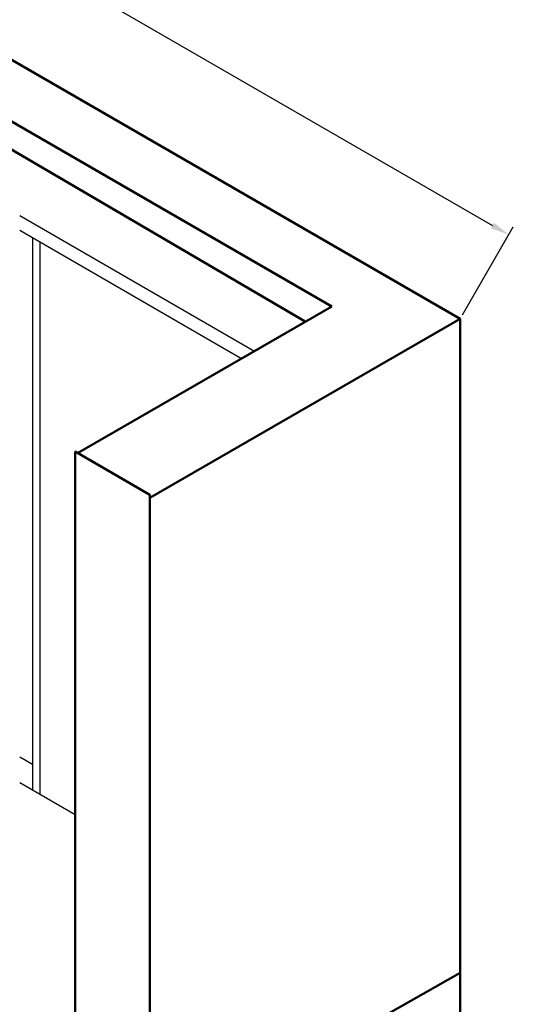
# Model space of a CAD drawing. Units: inches. Extents: x 5770 to 11891, y 3254 to 6808.
# Tile 13 of 15: x 6073 to 6140, y 3357 to 3489. Entities that reach past the tile are written whole.
import ezdxf

# ---------------------------------------------------------------- set-up
doc = ezdxf.new("R2010")
doc.units = ezdxf.units.IN
for name, color, linetype, lineweight in [('A-ANNO-DIMS', 2, 'Continuous', 18), ('A-DOOR', 4, 'Continuous', 25), ('A-WALL', 7, 'Continuous', 50)]:
    doc.layers.add(name, color=color, linetype=linetype, lineweight=lineweight)
doc.styles.get("Standard").update_dxf_attribs({"font": 'arial.ttf'})
doc.dimstyles.new('ISO-25', dxfattribs={"dimtxt": 2.5, "dimasz": 2.5, "dimexe": 1.25, "dimexo": 0.625, "dimtad": 1, "dimdec": 0, "dimlunit": 3, "dimtxsty": 'Standard', "dimcen": 2.5, "dimadec": 0, "dimazin": 0, "dimtfac": 1, "dimtdec": 0, "dimtmove": 0, "dimatfit": 3, "dimfxl": 1, "dimarcsym": 0})

# ---------------------------------------------------------------- blocks, each defined once
blk = doc.blocks.new('*D7')
at = {"layer": 'A-ANNO-DIMS', "color": 0, "lineweight": -2, "transparency": 16777216}
for p, q in [((5959.63, 3549.37), (5966.46, 3561.21)), ((5968, 3558.88), (6136.88, 3461.38)), ((6132.83, 3449.37), (6139.67, 3461.21))]:
    blk.add_line(p, q, dxfattribs=at)
at = {"layer": 'A-ANNO-DIMS', "color": 0, "transparency": 16777216}
for points in [[(5968.21, 3559.24), (5967.79, 3558.51), (5965.84, 3560.13)], [(6137.08, 3461.74), (6136.67, 3461.01), (6139.04, 3460.13)]]:
    blk.add_solid(points, dxfattribs=at)
at = {"layer": 'Defpoints', "color": 0, "transparency": 16777216}
for p in [(5959.31, 3548.83), (6139.04, 3460.13), (6132.52, 3448.83)]:
    blk.add_point(p, dxfattribs=at)
at = {"layer": 'A-ANNO-DIMS', "color": 0, "transparency": 16777216, "insert": (6061.62, 3507.02), "char_height": 2.5, "attachment_point": 5, "rotation": 330}
blk.add_mtext('16\'-8"', dxfattribs=at)

msp = doc.modelspace()

# ---------------------------------------------------------------- linework, layer by layer
at = {"layer": 'A-DOOR'}
for p, q in [((6073.26, 3462.72), (6104.85, 3444.48)), ((6073.26, 3460.72), (6103.12, 3443.48)), ((6074.99, 3459.72), (6074.99, 3385.42)), ((6075.98, 3459.15), (6075.98, 3384.85)), ((6074.99, 3388.83), (6073.26, 3389.83)), ((6073.26, 3386.42), (6080.71, 3382.12))]:
    msp.add_line(p, q, dxfattribs=at)
at = {"layer": 'A-WALL'}
for p, q in [((5959.31, 3548.83), (6132.52, 3448.83)), ((5959.31, 3540.51), (6115.24, 3450.48)), ((5974.02, 3529.02), (6111.68, 3448.43)), ((6081.05, 3430.74), (6115.24, 3450.48)), ((6132.52, 3448.83), (6090.78, 3424.73)), ((6132.52, 3448.83), (6132.52, 3360.83)), ((6132.52, 3448.83), (6132.52, 3352.22)), ((6080.71, 3430.94), (6080.71, 3342.94)), ((6090.78, 3425.13), (6080.71, 3430.94)), ((6090.78, 3425.13), (6090.78, 3337.13)), ((6132.52, 3360.83), (6090.78, 3337.13))]:
    msp.add_line(p, q, dxfattribs=at)

# ---------------------------------------------------------------- dimensions: what is measured, and where the dimension line sits
at = {"layer": 'A-ANNO-DIMS'}
dim = msp.add_linear_dim(base=(6139.04, 3460.13), p1=(5959.31, 3548.83), p2=(6132.52, 3448.83), angle=330, dimstyle='ISO-25', override={"dimclrd": 0, "dimclre": 0, "dimclrt": 0}, dxfattribs=at)
dim.commit()
dim.dimension.update_dxf_attribs({"geometry": '*D7', "text_midpoint": (6060.67, 3505.37), "dimtype": 161})

doc.saveas('drawing.dxf')
